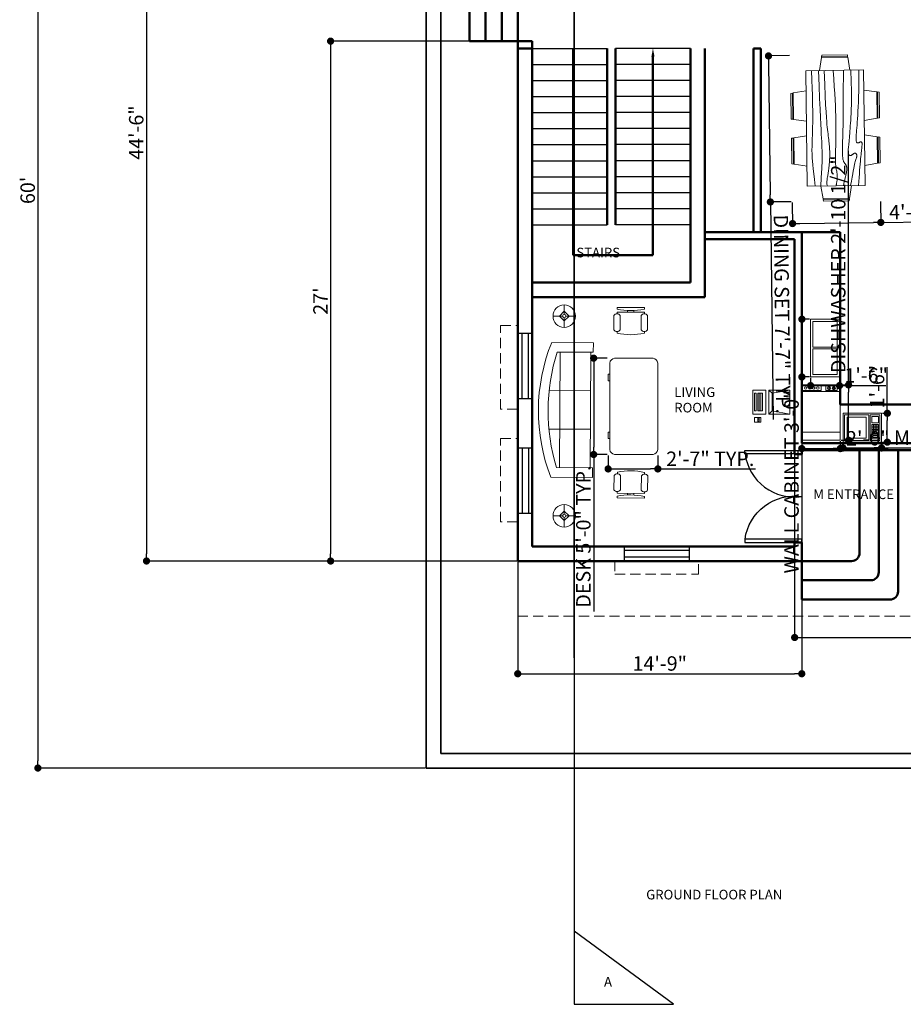
# Model space of a CAD drawing. Units: inches. Extents: x 2050 to 6806, y 2092 to 5743.
# Tile 1 of 8: x 2050 to 2600, y 2092 to 2706. Entities that reach past the tile are written whole.
import ezdxf

# ---------------------------------------------------------------- set-up
doc = ezdxf.new("R2010")
doc.units = ezdxf.units.IN
doc.linetypes.add('HIDDEN', pattern=[9.525, 6.35, -3.175])
for name, color, linetype, lineweight in [('A-ANNO-DIMS', 2, 'Continuous', 18), ('A-ANNO-SYMB', 1, 'Continuous', 25), ('A-ANNO-TEXT', 7, 'Continuous', 25), ('A-AREA-IDEN', 7, 'Continuous', 18), ('A-DOOR', 2, 'Continuous', 25), ('A-FLOR-FIXT', 4, 'Continuous', 18), ('A-FLOR-OVHD', 30, 'HIDDEN', 18), ('A-FLOR-STRS', 3, 'Continuous', 25), ('A-FURN', 5, 'Continuous', 18), ('A-GLAZ', 6, 'Continuous', 25), ('A-WALL', 7, 'Continuous', 50), ('C-PROP', 90, 'Continuous', 35)]:
    doc.layers.add(name, color=color, linetype=linetype, lineweight=lineweight)
doc.styles.get("Standard").update_dxf_attribs({"font": 'arial.ttf'})
doc.dimstyles.new('ISO-25', dxfattribs={"dimtxt": 9, "dimasz": 4.5, "dimexe": 1.25, "dimexo": 0.625, "dimtad": 1, "dimdec": 1, "dimlunit": 4, "dimtxsty": 'Standard', "dimblk": 'DOT', "dimcen": 2.5, "dimadec": 0, "dimazin": 0, "dimtfac": 1, "dimtdec": 1, "dimtmove": 0, "dimatfit": 3, "dimldrblk": 'ARCHTICK', "dimfxl": 1, "dimarcsym": 0})

# ---------------------------------------------------------------- blocks, each defined once
blk = doc.blocks.new('Dining Set - 36 x 72 in.')
for p, q in [((-22.2343, 26.00059), (-23.4847, 17.99762)), ((-22.2304, 26), (-5.7608, 26)), ((-22, 27.5), (-22.1562, 26.50042)), ((-5.8416, 26.5), (-22.1534, 26.5)), ((-22, 27.5), (-6, 27.5)), ((-5.8437, 26.49966), (-6, 27.5)), ((-4.5152, 17.99762), (-5.7655, 25.99926)), ((5.7657, 26.00059), (4.5153, 17.99762)), ((5.7696, 26), (22.2392, 26)), ((6, 27.5), (5.8438, 26.50042)), ((22.1584, 26.5), (5.8466, 26.5)), ((6, 27.5), (22, 27.5)), ((22.1563, 26.49966), (22, 27.5)), ((23.4848, 17.99762), (22.2345, 25.99926)), ((36, 18), (-36, 18)), ((-36, 18), (-36, -18)), ((36, -18), (36, 18)), ((-45.5, 8), (-44.5004, 8.15617)), ((-45.5, 8), (-45.5, -8)), ((-44.5, -8.15843), (-44.5, 8.15338)), ((-44.0006, 8.23428), (-35.9976, 9.48474)), ((-44, 8.23041), (-44, -8.23915)), ((44.0006, 8.23428), (35.9976, 9.48474)), ((44, 8.23041), (44, -8.23915)), ((44.5, -8.15843), (44.5, 8.15338)), ((45.5, 8), (44.5005, 8.15617)), ((45.5, 8), (45.5, -8)), ((-44.4997, -8.15631), (-45.5, -8)), ((-35.9976, -9.48476), (-43.9993, -8.2345)), ((35.9976, -9.48476), (43.9993, -8.2345)), ((44.4997, -8.15631), (45.5, -8)), ((-36, -18), (36, -18)), ((-22.2343, -26.0006), (-23.4847, -17.99762)), ((-4.5152, -17.99762), (-5.7655, -25.99928)), ((5.7657, -26.0006), (4.5153, -17.99762)), ((23.4848, -17.99762), (22.2345, -25.99928)), ((-22.2304, -26), (-5.7608, -26)), ((-22, -27.5), (-22.1562, -26.50044)), ((-5.8416, -26.5), (-22.1534, -26.5)), ((-22, -27.5), (-6, -27.5)), ((-5.8437, -26.49967), (-6, -27.5)), ((5.7696, -26), (22.2392, -26)), ((6, -27.5), (5.8438, -26.50044)), ((22.1584, -26.5), (5.8466, -26.5)), ((6, -27.5), (22, -27.5)), ((22.1563, -26.49967), (22, -27.5))]:
    blk.add_line(p, q)
for points in [[(-36, 15), (-31.1772, 14.97754), (-26.8079, 14.91406), (-22.8538, 14.81543), (-19.276, 14.6875), (-16.0362, 14.53613), (-13.0957, 14.36718), (-10.4159, 14.18652), (-7.9583, 14), (-5.6904, 13.81315), (-3.6035, 13.63021), (-1.6954, 13.45508), (0.0365, 13.29166), (1.5945, 13.14388), (2.9811, 13.01562), (4.1988, 12.9108), (5.25, 12.83333), (6.1393, 12.78613), (6.8802, 12.76823), (7.4883, 12.77767), (7.9792, 12.8125), (8.3685, 12.87077), (8.6719, 12.95052), (8.9049, 13.0498), (9.0833, 13.16666), (9.2205, 13.29899), (9.3216, 13.44401), (9.3895, 13.59879), (9.4271, 13.76041), (9.4373, 13.92594), (9.4232, 14.09245), (9.3875, 14.257), (9.3333, 14.41666), (9.2638, 14.56917), (9.1836, 14.71484), (9.0975, 14.85465), (9.0104, 14.98958), (8.9272, 15.1206), (8.8529, 15.2487), (8.7922, 15.37483), (8.75, 15.5), (8.7305, 15.62467), (8.7344, 15.74739), (8.7617, 15.86621), (8.8125, 15.97916), (8.8867, 16.08431), (8.9844, 16.17968), (9.1055, 16.26334), (9.25, 16.33333), (9.4189, 16.38802), (9.6172, 16.42708), (9.8506, 16.45052), (10.125, 16.45833), (10.4463, 16.45052), (10.8203, 16.42708), (11.2529, 16.38802), (11.75, 16.33333), (12.3184, 16.26318), (12.9694, 16.17838), (13.7151, 16.07991), (14.5677, 15.96875), (15.5395, 15.84586), (16.6426, 15.71224), (17.8893, 15.56884), (19.2917, 15.41666), (20.859, 15.25667), (22.5879, 15.08984), (24.4721, 14.91715), (26.5052, 14.73958), (28.6809, 14.5581), (30.9929, 14.3737), (33.4347, 14.18733), (36, 14)], [(-36, 10), (-28.9766, 10.14274), (-23.1725, 10.20442), (-18.4241, 10.19775), (-14.5677, 10.13541), (-11.4399, 10.03011), (-8.877, 9.89453), (-6.7154, 9.74137), (-4.7917, 9.58333), (-2.9698, 9.43082), (-1.2246, 9.28515), (0.4415, 9.14534), (2.026, 9.01041), (3.5266, 8.87939), (4.9408, 8.7513), (6.266, 8.62516), (7.5, 8.5), (8.6411, 8.37549), (9.6914, 8.2539), (10.6538, 8.13818), (11.5312, 8.03125), (12.3267, 7.93603), (13.043, 7.85547), (13.6831, 7.79248), (14.25, 7.75), (14.7471, 7.7303), (15.1797, 7.73307), (15.5537, 7.75732), (15.875, 7.80208), (16.1494, 7.86637), (16.3828, 7.94922), (16.5811, 8.04964), (16.75, 8.16666), (16.8944, 8.29915), (17.0143, 8.44531), (17.1089, 8.60319), (17.1771, 8.77083), (17.218, 8.94629), (17.2305, 9.1276), (17.2137, 9.31282), (17.1667, 9.5), (17.0895, 9.6875), (16.987, 9.875), (16.8649, 10.0625), (16.7292, 10.25), (16.5856, 10.4375), (16.4401, 10.625), (16.2985, 10.8125), (16.1667, 11), (16.05, 11.18733), (15.9518, 11.3737), (15.8752, 11.5581), (15.8229, 11.73958), (15.798, 11.91715), (15.8034, 12.08984), (15.842, 12.25667), (15.9167, 12.41666), (16.0295, 12.56836), (16.1784, 12.70833), (16.3605, 12.83268), (16.5729, 12.9375), (16.8127, 13.01888), (17.0768, 13.07291), (17.3625, 13.0957), (17.6667, 13.08333), (17.9894, 13.03312), (18.3418, 12.94726), (18.7382, 12.82918), (19.1927, 12.68229), (19.7195, 12.51001), (20.3327, 12.31575), (21.0465, 12.10294), (21.875, 11.875), (22.8357, 11.63354), (23.959, 11.37304), (25.2786, 11.08618), (26.8282, 10.76562), (28.6414, 10.40405), (30.752, 9.99414), (33.1936, 9.52856), (36, 9)], [(-36, 5.5), (-30.7157, 5.3348), (-26.069, 5.20963), (-21.9946, 5.11767), (-18.4271, 5.05208), (-15.3009, 5.00602), (-12.5508, 4.97265), (-10.1112, 4.94515), (-7.9167, 4.91666), (-5.909, 4.88167), (-4.0586, 4.83984), (-2.3429, 4.79215), (-0.7396, 4.73958), (0.7739, 4.6831), (2.22, 4.6237), (3.6213, 4.56233), (5, 4.5), (6.373, 4.43782), (7.7344, 4.3776), (9.0723, 4.32129), (10.375, 4.27083), (11.6309, 4.22819), (12.8281, 4.19531), (13.9551, 4.17415), (15, 4.16666), (15.954, 4.17448), (16.819, 4.19791), (17.6001, 4.23698), (18.3021, 4.29166), (18.9299, 4.36198), (19.4883, 4.44791), (19.9823, 4.54948), (20.4167, 4.66666), (20.7969, 4.79899), (21.1302, 4.94401), (21.4245, 5.09879), (21.6875, 5.26041), (21.9271, 5.42594), (22.1511, 5.59245), (22.3672, 5.757), (22.5834, 5.91666), (22.8065, 6.06868), (23.0404, 6.21093), (23.2879, 6.34147), (23.5521, 6.45833), (23.8358, 6.55957), (24.142, 6.64323), (24.4735, 6.70735), (24.8334, 6.75), (25.2235, 6.76969), (25.642, 6.76692), (26.0858, 6.74267), (26.5521, 6.69791), (27.0379, 6.63362), (27.5404, 6.55078), (28.0565, 6.45036), (28.5834, 6.33333), (29.1242, 6.19987), (29.7071, 6.04687), (30.3661, 5.87044), (31.1354, 5.66666), (32.0493, 5.43164), (33.142, 5.16146), (34.4475, 4.85221), (36, 4.5)], [(-36, -1), (-30.7915, -0.6591), (-26.0195, -0.38216), (-21.6519, -0.16284), (-17.6563, 0.00521), (-14.0005, 0.12833), (-10.6523, 0.21289), (-7.5796, 0.26522), (-4.75, 0.29166), (-2.134, 0.29793), (0.2878, 0.28711), (2.5317, 0.26163), (4.6146, 0.22396), (6.5529, 0.17651), (8.3633, 0.12174), (10.0623, 0.06209), (11.6667, 0), (13.1899, -0.06201), (14.6341, -0.1211), (15.9982, -0.17432), (17.2813, -0.21875), (18.4823, -0.25147), (19.6003, -0.26953), (20.6343, -0.27002), (21.5834, -0.25), (22.4481, -0.20768), (23.2357, -0.14584), (23.9549, -0.06836), (24.6146, 0.02083), (25.2235, 0.11784), (25.7904, 0.21875), (26.3241, 0.31966), (26.8334, 0.41666), (27.3265, 0.50618), (27.8099, 0.58593), (28.2894, 0.65397), (28.7709, 0.70833), (29.2601, 0.74707), (29.763, 0.76823), (30.2855, 0.76985), (30.8334, 0.75), (31.4088, 0.70784), (31.9994, 0.64713), (32.589, 0.57275), (33.1615, 0.48958), (33.7008, 0.4025), (34.1908, 0.3164), (34.6153, 0.23616), (34.9584, 0.16666), (35.2099, 0.11165), (35.3848, 0.07031), (35.504, 0.04069), (35.5886, 0.02083), (35.6594, 0.00879), (35.7377, 0.0026), (35.8442, 0.00032), (36, 0)], [(-36, -6.5), (-27.1843, -6.31267), (-20.084, -6.1263), (-14.469, -5.9419), (-10.1094, -5.76042), (-6.7752, -5.58285), (-4.2363, -5.41016), (-2.2629, -5.24333), (-0.625, -5.08334), (0.8708, -4.93099), (2.2715, -4.78646), (3.5872, -4.64974), (4.8281, -4.52084), (6.0046, -4.39974), (7.127, -4.28646), (8.2053, -4.18099), (9.25, -4.08334), (10.2705, -3.99382), (11.2734, -3.91407), (12.2647, -3.84603), (13.25, -3.79167), (14.2354, -3.75293), (15.2266, -3.73177), (16.2295, -3.73015), (17.25, -3.75), (18.2912, -3.79248), (19.3451, -3.85547), (20.4009, -3.93604), (21.4479, -4.03125), (22.4754, -4.13819), (23.4727, -4.25391), (24.4289, -4.37549), (25.3334, -4.5), (26.1785, -4.62492), (26.9694, -4.74935), (27.7145, -4.87281), (28.4219, -4.99479), (29.1, -5.11483), (29.7572, -5.23242), (30.4016, -5.34709), (31.0417, -5.45834), (31.6837, -5.56437), (32.3262, -5.65821), (32.9658, -5.73153), (33.599, -5.77604), (34.2224, -5.78345), (34.8327, -5.74545), (35.4264, -5.65373), (36, -5.5)], [(-36, -10), (-26.4022, -9.81299), (-18.4675, -9.62891), (-11.9839, -9.45069), (-6.7396, -9.28125), (-2.5226, -9.12354), (0.8789, -8.98047), (3.6769, -8.85498), (6.0833, -8.75), (8.2767, -8.66765), (10.3021, -8.60677), (12.1712, -8.56543), (13.8958, -8.54167), (15.4876, -8.53353), (16.9583, -8.53907), (18.3197, -8.55632), (19.5834, -8.58334), (20.7616, -8.61841), (21.8685, -8.66081), (22.9188, -8.71004), (23.9271, -8.76563), (24.9081, -8.82707), (25.8763, -8.89388), (26.8465, -8.96558), (27.8334, -9.04167), (28.8474, -9.12118), (29.8828, -9.20117), (30.93, -9.27824), (31.9792, -9.34896), (33.0205, -9.40991), (34.0443, -9.45768), (35.0407, -9.48885), (36, -9.5)], [(-36, -14.5), (-30.0881, -14.33513), (-25.0332, -14.21224), (-20.7312, -14.12647), (-17.0781, -14.07292), (-13.97, -14.04671), (-11.3027, -14.04297), (-8.9724, -14.05681), (-6.875, -14.08334), (-4.9224, -14.11833), (-3.0905, -14.16016), (-1.3709, -14.20785), (0.2448, -14.26042), (1.7647, -14.3169), (3.1973, -14.3763), (4.5507, -14.43767), (5.8333, -14.5), (7.0554, -14.5621), (8.235, -14.62175), (9.3922, -14.67652), (10.5469, -14.72396), (11.7192, -14.76164), (12.929, -14.78711), (14.1965, -14.79794), (15.5417, -14.79167), (16.9933, -14.76424), (18.6152, -14.70508), (20.4804, -14.60197), (22.6615, -14.44271), (25.2312, -14.21509), (28.2624, -13.9069), (31.8277, -13.50594), (36, -13)]]:
    blk.add_lwpolyline(points)
blk = doc.blocks.new('Microwave')
for p, q in [((18, 10), (22, 10)), ((22, 9), (18, 9)), ((18, 8), (22, 8)), ((22, 7), (18, 7)), ((19, 7), (19, 11)), ((19, 6), (19, 7)), ((20, 11), (20, 7)), ((20, 7), (20, 6)), ((21, 7), (21, 11)), ((20, 6), (18, 6))]:
    blk.add_line(p, q)
for points in [[(0, 0), (0, 18), (24, 18), (24, 0)], [(1, 1), (1, 17), (16, 17), (16, 1)], [(2.5, 2.5), (2.5, 15.5), (14.5, 15.5), (14.5, 2.5)], [(17, 1), (17, 17), (23, 17), (23, 1)], [(18, 12), (18, 16), (22, 16), (22, 12)], [(18, 2), (18, 11), (22, 11), (22, 2)], [(18.5, 4.5), (18.5, 5.5), (21.5, 5.5), (21.5, 4.5)], [(18.5, 3), (18.5, 4), (21.5, 4), (21.5, 3)]]:
    blk.add_lwpolyline(points, close=True)
blk = doc.blocks.new('Dishwasher')
for p, q in [((16, 32.5), (16.75, 32.5)), ((16.5, 32), (16.2942, 31.7942)), ((16.3156, 33.1843), (16.5, 33)), ((17, 32.75), (17, 33.5)), ((17, 32.25), (17, 31.5)), ((18, 32.5), (17.25, 32.5)), ((17.5, 33), (17.6938, 33.1938)), ((17.7061, 31.7939), (17.5, 32)), ((19, 32.5), (19.75, 32.5)), ((19.5, 32), (19.2942, 31.7942)), ((19.3156, 33.1843), (19.5, 33)), ((20, 32.75), (20, 33.5)), ((20, 32.25), (20, 31.5)), ((21, 32.5), (20.25, 32.5)), ((20.5, 33), (20.6938, 33.1938)), ((20.7061, 31.7939), (20.5, 32)), ((24, 30.5), (0, 30.5)), ((0, 5), (24, 5))]:
    blk.add_line(p, q)
for points in [[(0, 0), (0, 34.5), (24, 34.5), (24, 0)], [(0.5, 31), (0.5, 34), (12, 34), (12, 31)], [(15, 31), (15, 34), (22, 34), (22, 31)]]:
    blk.add_lwpolyline(points, close=True)
for centre, radius in [((2.5, 32.5), 0.75), ((5, 32.5), 0.75), ((7.5, 32.5), 0.75), ((10, 32.5), 0.75), ((17, 32.5), 1), ((20, 32.5), 1)]:
    blk.add_circle(centre, radius)
blk = doc.blocks.new('Wall Cabinet - 18 x 36 in front')
for p, q in [((17.5, -1.5), (17.5, -16.5)), ((18.5, -16.5), (18.5, -1.5))]:
    blk.add_line(p, q)
blk.add_lwpolyline([(0, -18), (0, 0), (36, 0), (36, -18)], close=True)
for points in [[(17.5, -16.5), (1.5, -16.5), (1.5, -1.5), (17.5, -1.5)], [(18.5, -1.5), (34.5, -1.5), (34.5, -16.5), (18.5, -16.5)]]:
    blk.add_lwpolyline(points)
blk = doc.blocks.new('Sofa - Roundback 7 ft.')
for p, q in [((-36.000027, -34), (-36.000027, -11.4696)), ((-12.00002, -32.4421), (-12.00003, -6.5971)), ((11.99997, -32.4421), (11.99998, -6.5971)), ((35.99998, -34), (35.99998, -11.4696)), ((-35.999844, -13.3819), (35.9998, -13.3819)), ((-36.000027, -32.4421), (35.99998, -32.4421))]:
    blk.add_line(p, q)
for points in [[(-36.000027, -34), (-42.000027, -34), (-42.000027, -8)], [(41.99998, -8), (41.99998, -34), (35.99998, -34)]]:
    blk.add_lwpolyline(points)
for centre, radius, start, end in [((0, -114.25), 114.25, 68.43141, 111.5686), ((-0.00001, -127.1968), 121.1968, 72.72033, 107.2797)]:
    blk.add_arc(centre, radius, start, end)
blk = doc.blocks.new('Desk - 30 x 60 in.')
for p, q in [((-26.999995, 0), (26.999995, 0)), ((-29.999995, -27), (-29.999995, -3)), ((29.999995, -3), (29.999995, -27)), ((26.999995, -30), (-26.999995, -30)), ((-20.000005, -30), (-20.000005, -31)), ((-16.000005, -31), (-16.000005, -30)), ((15.999995, -31), (15.999995, -30)), ((19.999995, -30), (19.999995, -31)), ((-20.000005, -31), (-16.000005, -31)), ((19.999995, -31), (15.999995, -31))]:
    blk.add_line(p, q)
for centre, start, end in [((-26.499995, -3.5), 98.1301, 171.8699), ((26.499995, -3.5), 8.130102, 81.8699), ((-26.499995, -26.5), 188.1301, 261.8699), ((26.499995, -26.5), 278.1301, 351.8699)]:
    blk.add_arc(centre, 3.535534, start, end)
blk = doc.blocks.new('Chair - Desk')
for p, q in [((-8.5, 0), (-8.5, -1)), ((-8.5, 0), (8.5, 0)), ((8.5, 0), (8.5, -1)), ((-10.5, -5), (-10.5, -14)), ((-8.5, -3), (-8.5, -4)), ((-8.5, -3), (8.5, -3)), ((-6.5, -14), (-6.5, -5)), ((-2, -3), (-2, -1.9355)), ((2, -1.9576), (2, -3)), ((6.5, -5), (6.5, -14)), ((8.5, -3), (8.5, -4)), ((10.5, -14), (10.5, -5)), ((-8.5, -15), (-8.5, -16)), ((8.5, -15), (8.5, -16))]:
    blk.add_line(p, q)
for centre, radius, start, end in [((-8.5, -6.5), 2.5, 36.8699, 143.1301), ((0, 34.625), 36.625, 256.5803, 283.4197), ((8.5, -6.5), 2.5, 36.8699, 143.1301), ((-8.5, -12.5), 2.5, 216.8699, 323.1301), ((0, 19.625), 36.625, 256.5803, 283.4197), ((8.5, -12.5), 2.5, 216.8699, 323.1301)]:
    blk.add_arc(centre, radius, start, end)
blk = doc.blocks.new('Lamp - Table')
for p, q in [((0, 7), (0, 1)), ((-1, 0), (-7, 0)), ((0, 3), (-3, 0)), ((-3, 0), (0, -3)), ((3, 0), (0, 3)), ((0, -3), (3, 0)), ((1, 0), (7, 0)), ((0, -1), (0, -7))]:
    blk.add_line(p, q)
for radius in [7, 1]:
    blk.add_circle((0, 0), radius)
blk = doc.blocks.new('Computer Terminal')
for p, q in [((-10, 11.5), (5, 11.5)), ((-8, 0.5), (-10, 11.5)), ((-10, -1.5), (-10, 11.5)), ((5, 11.5), (3, 0.5)), ((5, 11.5), (5, -1.5)), ((-10, -1.5), (-8, 0.5)), ((3, 0.5), (-8, 0.5)), ((3, 0.5), (5, -1.5)), ((5, -1.5), (-10, -1.5)), ((-10, -11.5), (-10, -3.5)), ((-10, -3.5), (5, -3.5)), ((-8, -5.5), (-8, -8.5)), ((3, -5.5), (-8, -5.5)), ((3, -8.5), (3, -5.5)), ((5, -3.5), (5, -11.5)), ((5, -11.5), (-10, -11.5)), ((3, -6.5), (-8, -6.5)), ((-8, -7.5), (3, -7.5)), ((-8, -8.5), (3, -8.5)), ((-8, -9.5), (-8, -10.5)), ((3, -9.5), (-8, -9.5)), ((-8, -10.5), (3, -10.5)), ((3, -10.5), (3, -9.5)), ((10, -6.5), (7, -6.5)), ((7, -6.5), (7, -10.5)), ((7, -10.5), (10, -10.5)), ((9.5, -7.5), (7.5, -7.5)), ((7.5, -7.5), (7.5, -8.5)), ((7.5, -8.5), (9.5, -8.5)), ((8.5, -7.5), (8.5, -8.5)), ((9.5, -8.5), (9.5, -7.5)), ((10, -10.5), (10, -6.5))]:
    blk.add_line(p, q)
blk = doc.blocks.new('_Dot')
at = {"color": 0, "linetype": 'ByBlock', "lineweight": -2}
blk.add_line((-0.5, 0), (-1, 0), dxfattribs=at)
at = {"color": 0, "linetype": 'ByBlock', "const_width": 0.5}
blk.add_lwpolyline([(-0.25, 0, 1), (0.25, 0, 1)], format="xyb", close=True, dxfattribs=at)
blk = doc.blocks.new('*D27')
at = {"layer": 'A-ANNO-DIMS', "color": 0, "lineweight": -2, "transparency": 16777216}
for p, q in [((2302.28, 2959.24), (2059.63, 2959.24)), ((2060.88, 2954.74), (2060.88, 2243.74)), ((2302.28, 2239.24), (2059.63, 2239.24))]:
    blk.add_line(p, q, dxfattribs=at)
at = {"layer": 'Defpoints', "color": 0, "transparency": 16777216}
for p in [(2302.91, 2959.24), (2060.88, 2239.24), (2302.91, 2239.24)]:
    blk.add_point(p, dxfattribs=at)
at = {"layer": 'A-ANNO-DIMS', "color": 0, "lineweight": -2, "transparency": 16777216, "xscale": 4.5, "yscale": 4.5, "zscale": 4.5}
for p, rotation in [((2060.88, 2959.24), 90), ((2060.88, 2239.24), 270)]:
    blk.add_blockref('_Dot', p, dxfattribs=dict(at, rotation=rotation))
at = {"layer": 'A-ANNO-DIMS', "color": 0, "transparency": 16777216, "insert": (2055.66, 2599.24), "char_height": 9, "attachment_point": 5, "rotation": 90}
blk.add_mtext("60'", dxfattribs=at)
blk = doc.blocks.new('_ArchTick')
at = {"color": 0, "linetype": 'ByBlock', "const_width": 0.15}
blk.add_lwpolyline([(-0.5, -0.5), (0.5, 0.5)], dxfattribs=at)
blk = doc.blocks.new('*D28')
at = {"layer": 'A-ANNO-DIMS', "color": 0, "lineweight": -2, "transparency": 16777216}
for p, q in [((2359.28, 2902.24), (2127.3, 2902.24)), ((2128.55, 2897.74), (2128.55, 2372.74)), ((2359.28, 2368.24), (2127.3, 2368.24))]:
    blk.add_line(p, q, dxfattribs=at)
at = {"layer": 'Defpoints', "color": 0, "transparency": 16777216}
for p in [(2359.91, 2902.24), (2128.55, 2368.24), (2359.91, 2368.24)]:
    blk.add_point(p, dxfattribs=at)
at = {"layer": 'A-ANNO-DIMS', "color": 0, "lineweight": -2, "transparency": 16777216, "xscale": 4.5, "yscale": 4.5, "zscale": 4.5}
for p, rotation in [((2128.55, 2902.24), 90), ((2128.55, 2368.24), 270)]:
    blk.add_blockref('_Dot', p, dxfattribs=dict(at, rotation=rotation))
at = {"layer": 'A-ANNO-DIMS', "color": 0, "transparency": 16777216, "insert": (2123.33, 2635.24), "char_height": 9, "attachment_point": 5, "rotation": 90}
blk.add_mtext('44\'-6"', dxfattribs=at)
blk = doc.blocks.new('*D30')
at = {"layer": 'A-ANNO-DIMS', "color": 0, "lineweight": -2, "transparency": 16777216}
for p, q in [((2359.28, 2692.24), (2242.04, 2692.24)), ((2243.29, 2687.74), (2243.29, 2372.74)), ((2359.28, 2368.24), (2242.04, 2368.24))]:
    blk.add_line(p, q, dxfattribs=at)
at = {"layer": 'Defpoints', "color": 0, "transparency": 16777216}
for p in [(2359.91, 2692.24), (2243.29, 2368.24), (2359.91, 2368.24)]:
    blk.add_point(p, dxfattribs=at)
at = {"layer": 'A-ANNO-DIMS', "color": 0, "lineweight": -2, "transparency": 16777216, "xscale": 4.5, "yscale": 4.5, "zscale": 4.5}
for p, rotation in [((2243.29, 2692.24), 90), ((2243.29, 2368.24), 270)]:
    blk.add_blockref('_Dot', p, dxfattribs=dict(at, rotation=rotation))
at = {"layer": 'A-ANNO-DIMS', "color": 0, "transparency": 16777216, "insert": (2238.15, 2530.24), "char_height": 9, "attachment_point": 5, "rotation": 90}
blk.add_mtext("27'", dxfattribs=at)
blk = doc.blocks.new('*D31')
at = {"layer": 'A-ANNO-DIMS', "color": 0, "lineweight": -2, "transparency": 16777216}
for p, q in [((2359.91, 2367.61), (2359.91, 2296.75)), ((2536.91, 2367.61), (2536.91, 2296.75)), ((2364.41, 2298), (2532.41, 2298))]:
    blk.add_line(p, q, dxfattribs=at)
at = {"layer": 'Defpoints', "color": 0, "transparency": 16777216}
for p in [(2359.91, 2368.24), (2536.91, 2368.24), (2536.91, 2298)]:
    blk.add_point(p, dxfattribs=at)
at = {"layer": 'A-ANNO-DIMS', "color": 0, "lineweight": -2, "transparency": 16777216, "xscale": 4.5, "yscale": 4.5, "zscale": 4.5, "rotation": 180}
blk.add_blockref('_Dot', (2359.91, 2298), dxfattribs=at)
at = {"layer": 'A-ANNO-DIMS', "color": 0, "lineweight": -2, "transparency": 16777216, "xscale": 4.5, "yscale": 4.5, "zscale": 4.5}
blk.add_blockref('_Dot', (2536.91, 2298), dxfattribs=at)
at = {"layer": 'A-ANNO-DIMS', "color": 0, "transparency": 16777216, "insert": (2448.41, 2303.22), "char_height": 9, "attachment_point": 5}
blk.add_mtext('14\'-9"', dxfattribs=at)
blk = doc.blocks.new('*D32')
at = {"layer": 'A-ANNO-DIMS', "color": 0, "lineweight": -2, "transparency": 16777216}
for p, q in [((2532.41, 2436.47), (2532.47, 2319.32)), ((2821.91, 2436.61), (2821.97, 2319.47)), ((2536.97, 2320.57), (2817.47, 2320.71))]:
    blk.add_line(p, q, dxfattribs=at)
at = {"layer": 'Defpoints', "color": 0, "transparency": 16777216}
for p in [(2532.41, 2437.09), (2821.91, 2437.24), (2821.97, 2320.72)]:
    blk.add_point(p, dxfattribs=at)
at = {"layer": 'A-ANNO-DIMS', "color": 0, "lineweight": -2, "transparency": 16777216, "xscale": 4.5, "yscale": 4.5, "zscale": 4.5}
for p, rotation in [((2532.47, 2320.57), 180.0291193537901), ((2821.97, 2320.72), 0.029119353790171)]:
    blk.add_blockref('_Dot', p, dxfattribs=dict(at, rotation=rotation))
at = {"layer": 'A-ANNO-DIMS', "color": 0, "transparency": 16777216, "insert": (2677.21, 2331.81), "char_height": 9, "attachment_point": 5, "rotation": 0.02912}
blk.add_mtext('24\'-1{\\H1x;\\S1/2;}"', dxfattribs=at)
blk = doc.blocks.new('DOOR-750')
blk.add_lwpolyline([(28.97, 0), (26.83, 0), (26.83, 35.38), (28.97, 35.38)], close=True)
blk.add_arc((31.25, 4.42), 31.27, 98.12333, 188.12333)
blk = doc.blocks.new('DOOR-DOUBLE')
blk.add_lwpolyline([(35.38, 28.96), (35.38, 26.82), (0, 26.82), (0, 28.96)], close=True)
blk.add_lwpolyline([(35.38, 28.96), (35.38, 26.82), (0, 26.82), (0, 28.96)], close=True)
blk.add_arc((30.96, 31.24), 31.27, 188.12333, 278.12333)
blk.add_arc((30.96, 31.24), 31.27, 188.12333, 278.12333)
blk = doc.blocks.new('WIN-1050')
for p, q in [((0, 40.58), (9, 40.58)), ((2.5, 0), (2.5, 40.58)), ((6.5, 0), (6.5, 40.58)), ((0, 0), (9, 0))]:
    blk.add_line(p, q)
blk = doc.blocks.new('SUNSHADE-A')
for p, q in [((0, 52.08), (10.45, 52.08)), ((10.45, 52.08), (10.45, 0)), ((10.45, 0), (0, 0))]:
    blk.add_line(p, q)
blk = doc.blocks.new('SUNSHADE-C')
for p, q in [((0, 8.26), (0, 0)), ((52.07, 0), (52.07, 8.25)), ((0, 0), (52.07, 0))]:
    blk.add_line(p, q)
blk = doc.blocks.new('*D93')
at = {"layer": 'A-ANNO-DIMS', "color": 0, "lineweight": -2, "transparency": 16777216}
for p, q in [((2529.19, 2683.19), (2514.92, 2683)), ((2516.23, 2678.52), (2517.28, 2596.53)), ((2530.36, 2592.19), (2516.09, 2592.01)), ((2517.34, 2592.03), (2519.07, 2456.43))]:
    blk.add_line(p, q, dxfattribs=at)
at = {"layer": 'Defpoints', "color": 0, "transparency": 16777216}
for p in [(2529.82, 2683.2), (2517.34, 2592.03), (2530.98, 2592.2)]:
    blk.add_point(p, dxfattribs=at)
at = {"layer": 'A-ANNO-DIMS', "color": 0, "lineweight": -2, "transparency": 16777216, "xscale": 4.5, "yscale": 4.5, "zscale": 4.5}
for p, rotation in [((2516.17, 2683.02), 90.73372649959308), ((2517.34, 2592.03), 270.733726499593)]:
    blk.add_blockref('_Dot', p, dxfattribs=dict(at, rotation=rotation))
at = {"layer": 'A-ANNO-DIMS', "color": 0, "transparency": 16777216, "insert": (2523.51, 2522.05), "char_height": 9, "attachment_point": 5, "rotation": 270.73373}
blk.add_mtext('DINING SET 7\'-7" TYP.', dxfattribs=at)
blk = doc.blocks.new('*D94')
at = {"layer": 'A-ANNO-DIMS', "color": 0, "lineweight": -2, "transparency": 16777216}
for p, q in [((2530.99, 2591.58), (2531.18, 2577.3)), ((2585.99, 2592.28), (2586.17, 2578.01)), ((2535.66, 2578.61), (2581.66, 2579.2)), ((2586.16, 2579.26), (2647.12, 2580.04))]:
    blk.add_line(p, q, dxfattribs=at)
at = {"layer": 'Defpoints', "color": 0, "transparency": 16777216}
for p in [(2530.98, 2592.2), (2585.98, 2592.91), (2586.16, 2579.26)]:
    blk.add_point(p, dxfattribs=at)
at = {"layer": 'A-ANNO-DIMS', "color": 0, "lineweight": -2, "transparency": 16777216, "xscale": 4.5, "yscale": 4.5, "zscale": 4.5}
for p, rotation in [((2531.16, 2578.55), 180.7337264995931), ((2586.16, 2579.26), 0.7337264995931003)]:
    blk.add_blockref('_Dot', p, dxfattribs=dict(at, rotation=rotation))
at = {"layer": 'A-ANNO-DIMS', "color": 0, "transparency": 16777216, "insert": (2618.82, 2584.8), "char_height": 9, "attachment_point": 5, "rotation": 0.73373}
blk.add_mtext('4\'-7" TYP.', dxfattribs=at)
blk = doc.blocks.new('*D97')
at = {"layer": 'A-ANNO-DIMS', "color": 0, "lineweight": -2, "transparency": 16777216}
for p, q in [((2415.62, 2494.64), (2405.99, 2494.64)), ((2407.24, 2490.14), (2407.24, 2439.14)), ((2415.62, 2434.64), (2405.99, 2434.64)), ((2407.24, 2434.64), (2407.24, 2336.75))]:
    blk.add_line(p, q, dxfattribs=at)
at = {"layer": 'Defpoints', "color": 0, "transparency": 16777216}
for p in [(2416.24, 2494.64), (2407.24, 2434.64), (2416.24, 2434.64)]:
    blk.add_point(p, dxfattribs=at)
at = {"layer": 'A-ANNO-DIMS', "color": 0, "lineweight": -2, "transparency": 16777216, "xscale": 4.5, "yscale": 4.5, "zscale": 4.5}
for p, rotation in [((2407.24, 2494.64), 90), ((2407.24, 2434.64), 270)]:
    blk.add_blockref('_Dot', p, dxfattribs=dict(at, rotation=rotation))
at = {"layer": 'A-ANNO-DIMS', "color": 0, "transparency": 16777216, "insert": (2401.96, 2383.45), "char_height": 9, "attachment_point": 5, "rotation": 90}
blk.add_mtext('DESK 5\'-0" TYP.', dxfattribs=at)
blk = doc.blocks.new('*D98')
at = {"layer": 'A-ANNO-DIMS', "color": 0, "lineweight": -2, "transparency": 16777216}
for p, q in [((2416.24, 2434.02), (2416.24, 2424.39)), ((2447.24, 2434.02), (2447.24, 2424.39)), ((2420.74, 2425.64), (2442.74, 2425.64)), ((2447.24, 2425.64), (2508, 2425.64))]:
    blk.add_line(p, q, dxfattribs=at)
at = {"layer": 'Defpoints', "color": 0, "transparency": 16777216}
for p in [(2416.24, 2434.64), (2447.24, 2434.64), (2447.24, 2425.64)]:
    blk.add_point(p, dxfattribs=at)
at = {"layer": 'A-ANNO-DIMS', "color": 0, "lineweight": -2, "transparency": 16777216, "xscale": 4.5, "yscale": 4.5, "zscale": 4.5, "rotation": 180}
blk.add_blockref('_Dot', (2416.24, 2425.64), dxfattribs=at)
at = {"layer": 'A-ANNO-DIMS', "color": 0, "lineweight": -2, "transparency": 16777216, "xscale": 4.5, "yscale": 4.5, "zscale": 4.5}
blk.add_blockref('_Dot', (2447.24, 2425.64), dxfattribs=at)
at = {"layer": 'A-ANNO-DIMS', "color": 0, "transparency": 16777216, "insert": (2479.87, 2430.79), "char_height": 9, "attachment_point": 5}
blk.add_mtext('2\'-7" TYP.', dxfattribs=at)
blk = doc.blocks.new('*D105')
at = {"layer": 'A-ANNO-DIMS', "color": 0, "lineweight": -2, "transparency": 16777216}
for p, q in [((2562.63, 2441.66), (2562.63, 2437.44)), ((2567.13, 2438.69), (2582.13, 2438.69)), ((2586.63, 2441.66), (2586.63, 2437.44)), ((2586.63, 2438.69), (2698.32, 2438.69))]:
    blk.add_line(p, q, dxfattribs=at)
at = {"layer": 'Defpoints', "color": 0, "transparency": 16777216}
for p in [(2562.63, 2442.29), (2586.63, 2442.29), (2586.63, 2438.69)]:
    blk.add_point(p, dxfattribs=at)
at = {"layer": 'A-ANNO-DIMS', "color": 0, "lineweight": -2, "transparency": 16777216, "xscale": 4.5, "yscale": 4.5, "zscale": 4.5, "rotation": 180}
blk.add_blockref('_Dot', (2562.63, 2438.69), dxfattribs=at)
at = {"layer": 'A-ANNO-DIMS', "color": 0, "lineweight": -2, "transparency": 16777216, "xscale": 4.5, "yscale": 4.5, "zscale": 4.5}
blk.add_blockref('_Dot', (2586.63, 2438.69), dxfattribs=at)
at = {"layer": 'A-ANNO-DIMS', "color": 0, "transparency": 16777216, "insert": (2644.72, 2443.97), "char_height": 9, "attachment_point": 5}
blk.add_mtext('MICROWAVE 2\'-0"', dxfattribs=at)
blk = doc.blocks.new('*D106')
at = {"layer": 'A-ANNO-DIMS', "color": 0, "lineweight": -2, "transparency": 16777216}
for p, q in [((2590.23, 2460.29), (2590.23, 2489.12)), ((2587.25, 2460.29), (2591.48, 2460.29)), ((2590.23, 2446.79), (2590.23, 2455.79)), ((2587.25, 2442.29), (2591.48, 2442.29))]:
    blk.add_line(p, q, dxfattribs=at)
at = {"layer": 'Defpoints', "color": 0, "transparency": 16777216}
for p in [(2586.63, 2460.29), (2590.23, 2460.29), (2586.63, 2442.29)]:
    blk.add_point(p, dxfattribs=at)
at = {"layer": 'A-ANNO-DIMS', "color": 0, "lineweight": -2, "transparency": 16777216, "xscale": 4.5, "yscale": 4.5, "zscale": 4.5}
for p, rotation in [((2590.23, 2460.29), 90), ((2590.23, 2442.29), 270)]:
    blk.add_blockref('_Dot', p, dxfattribs=dict(at, rotation=rotation))
at = {"layer": 'A-ANNO-DIMS', "color": 0, "transparency": 16777216, "insert": (2585.01, 2476.95), "char_height": 9, "attachment_point": 5, "rotation": 90}
blk.add_mtext('1\'-6"', dxfattribs=at)
blk = doc.blocks.new('*D107')
at = {"layer": 'A-ANNO-DIMS', "color": 0, "lineweight": -2, "transparency": 16777216}
for p, q in [((2566.08, 2477.99), (2566.08, 2623.89)), ((2561.53, 2477.99), (2567.33, 2477.99)), ((2566.08, 2447.99), (2566.08, 2473.49)), ((2561.53, 2443.49), (2567.33, 2443.49))]:
    blk.add_line(p, q, dxfattribs=at)
at = {"layer": 'Defpoints', "color": 0, "transparency": 16777216}
for p in [(2560.91, 2477.99), (2566.08, 2477.99), (2560.91, 2443.49)]:
    blk.add_point(p, dxfattribs=at)
at = {"layer": 'A-ANNO-DIMS', "color": 0, "lineweight": -2, "transparency": 16777216, "xscale": 4.5, "yscale": 4.5, "zscale": 4.5}
for p, rotation in [((2566.08, 2477.99), 90), ((2566.08, 2443.49), 270)]:
    blk.add_blockref('_Dot', p, dxfattribs=dict(at, rotation=rotation))
at = {"layer": 'A-ANNO-DIMS', "color": 0, "transparency": 16777216, "insert": (2560.81, 2553.19), "char_height": 9, "attachment_point": 5, "rotation": 90}
blk.add_mtext('DISHWASHER 2\'-10 1/2"', dxfattribs=at)
blk = doc.blocks.new('*D108')
at = {"layer": 'A-ANNO-DIMS', "color": 0, "lineweight": -2, "transparency": 16777216}
for p, q in [((2536.91, 2442.86), (2536.91, 2437.06)), ((2560.91, 2442.86), (2560.91, 2437.06)), ((2541.41, 2438.31), (2556.41, 2438.31)), ((2560.91, 2438.31), (2590.74, 2438.31))]:
    blk.add_line(p, q, dxfattribs=at)
at = {"layer": 'Defpoints', "color": 0, "transparency": 16777216}
for p in [(2536.91, 2443.49), (2560.91, 2443.49), (2560.91, 2438.31)]:
    blk.add_point(p, dxfattribs=at)
at = {"layer": 'A-ANNO-DIMS', "color": 0, "lineweight": -2, "transparency": 16777216, "xscale": 4.5, "yscale": 4.5, "zscale": 4.5, "rotation": 180}
blk.add_blockref('_Dot', (2536.91, 2438.31), dxfattribs=at)
at = {"layer": 'A-ANNO-DIMS', "color": 0, "lineweight": -2, "transparency": 16777216, "xscale": 4.5, "yscale": 4.5, "zscale": 4.5}
blk.add_blockref('_Dot', (2560.91, 2438.31), dxfattribs=at)
at = {"layer": 'A-ANNO-DIMS', "color": 0, "transparency": 16777216, "insert": (2578.07, 2443.53), "char_height": 9, "attachment_point": 5}
blk.add_mtext('2\'-0"', dxfattribs=at)
blk = doc.blocks.new('*D109')
at = {"layer": 'A-ANNO-DIMS', "color": 0, "lineweight": -2, "transparency": 16777216}
for p, q in [((2541.77, 2518.94), (2535.75, 2518.94)), ((2537, 2514.44), (2537, 2487.44)), ((2541.77, 2482.94), (2535.75, 2482.94)), ((2537, 2482.94), (2537, 2357.18))]:
    blk.add_line(p, q, dxfattribs=at)
at = {"layer": 'Defpoints', "color": 0, "transparency": 16777216}
for p in [(2542.4, 2518.94), (2537, 2482.94), (2542.4, 2482.94)]:
    blk.add_point(p, dxfattribs=at)
at = {"layer": 'A-ANNO-DIMS', "color": 0, "lineweight": -2, "transparency": 16777216, "xscale": 4.5, "yscale": 4.5, "zscale": 4.5}
for p, rotation in [((2537, 2518.94), 90), ((2537, 2482.94), 270)]:
    blk.add_blockref('_Dot', p, dxfattribs=dict(at, rotation=rotation))
at = {"layer": 'A-ANNO-DIMS', "color": 0, "transparency": 16777216, "insert": (2531.72, 2417.81), "char_height": 9, "attachment_point": 5, "rotation": 90}
blk.add_mtext('WALL CABINET 3\'-0"', dxfattribs=at)
blk = doc.blocks.new('*D110')
at = {"layer": 'A-ANNO-DIMS', "color": 0, "lineweight": -2, "transparency": 16777216}
for p, q in [((2542.4, 2482.32), (2542.4, 2476.29)), ((2560.4, 2482.32), (2560.4, 2476.29)), ((2546.9, 2477.54), (2555.9, 2477.54)), ((2560.4, 2477.54), (2589.22, 2477.54))]:
    blk.add_line(p, q, dxfattribs=at)
at = {"layer": 'Defpoints', "color": 0, "transparency": 16777216}
for p in [(2542.4, 2482.94), (2560.4, 2482.94), (2560.4, 2477.54)]:
    blk.add_point(p, dxfattribs=at)
at = {"layer": 'A-ANNO-DIMS', "color": 0, "lineweight": -2, "transparency": 16777216, "xscale": 4.5, "yscale": 4.5, "zscale": 4.5, "rotation": 180}
blk.add_blockref('_Dot', (2542.4, 2477.54), dxfattribs=at)
at = {"layer": 'A-ANNO-DIMS', "color": 0, "lineweight": -2, "transparency": 16777216, "xscale": 4.5, "yscale": 4.5, "zscale": 4.5}
blk.add_blockref('_Dot', (2560.4, 2477.54), dxfattribs=at)
at = {"layer": 'A-ANNO-DIMS', "color": 0, "transparency": 16777216, "insert": (2577.06, 2482.76), "char_height": 9, "attachment_point": 5}
blk.add_mtext('1\'-6"', dxfattribs=at)

msp = doc.modelspace()

# ---------------------------------------------------------------- linework, layer by layer
at = {"layer": 'A-ANNO-SYMB'}
for p, q in [((2395, 3128.67), (2395, 2091.98)), ((2395, 2307.82), (2395, 3128.67)), ((2456.98, 2091.98), (2395, 2137.51)), ((2395, 2091.98), (2456.98, 2091.98)), ((2456.98, 2091.98), (2456.98, 2091.98))]:
    msp.add_line(p, q, dxfattribs=at)
at = {"layer": 'A-FLOR-OVHD'}
for p, q in [((2359.91, 2368.24), (2359.91, 2333.88)), ((2359.91, 2333.88), (2608.94, 2333.88))]:
    msp.add_line(p, q, dxfattribs=at)
at = {"layer": 'A-FLOR-STRS'}
for p, q in [((2368.91, 2687.74), (2404.91, 2687.74)), ((2368.91, 2687.74), (2415.59, 2687.74)), ((2467.51, 2687.74), (2420.83, 2687.74)), ((2467.51, 2687.74), (2431.51, 2687.74)), ((2368.91, 2677.74), (2415.59, 2677.74)), ((2467.51, 2677.74), (2420.83, 2677.74)), ((2368.91, 2667.74), (2415.59, 2667.74)), ((2467.51, 2667.74), (2420.83, 2667.74)), ((2368.91, 2657.74), (2415.59, 2657.74)), ((2467.51, 2657.74), (2420.83, 2657.74)), ((2368.91, 2647.74), (2415.59, 2647.74)), ((2467.51, 2647.74), (2420.83, 2647.74)), ((2368.91, 2637.74), (2415.59, 2637.74)), ((2467.51, 2637.74), (2420.83, 2637.74)), ((2368.91, 2627.74), (2415.59, 2627.74)), ((2467.51, 2627.74), (2420.83, 2627.74)), ((2368.91, 2617.74), (2415.59, 2617.74)), ((2467.51, 2617.74), (2420.83, 2617.74)), ((2368.91, 2607.74), (2415.59, 2607.74)), ((2467.51, 2607.74), (2420.83, 2607.74)), ((2368.91, 2597.74), (2415.59, 2597.74)), ((2467.51, 2597.74), (2420.83, 2597.74)), ((2368.91, 2587.74), (2415.59, 2587.74)), ((2467.51, 2587.74), (2420.83, 2587.74)), ((2368.91, 2577.74), (2415.59, 2577.74)), ((2467.51, 2577.74), (2420.83, 2577.74)), ((2368.91, 2541.74), (2415.59, 2541.74))]:
    msp.add_line(p, q, dxfattribs=at)
at = {"layer": 'A-WALL'}
for p, q in [((2329.91, 2692.24), (2329.91, 2740.24)), ((2339.91, 2692.24), (2339.91, 2740.24)), ((2349.91, 2692.24), (2349.91, 2740.24)), ((2359.91, 2692.24), (2359.91, 2740.24)), ((2329.91, 2692.24), (2359.91, 2692.24)), ((2368.91, 2692.24), (2359.91, 2692.24)), ((2359.91, 2692.24), (2359.91, 2368.24)), ((2368.91, 2687.74), (2359.91, 2687.74)), ((2368.91, 2692.24), (2368.91, 2377.24)), ((2394.39, 2558.75), (2394.39, 2687.74)), ((2415.59, 2687.74), (2415.59, 2577.74)), ((2420.83, 2687.74), (2420.83, 2577.74)), ((2467.51, 2687.74), (2467.51, 2541.74)), ((2476.51, 2687.74), (2476.51, 2532.74)), ((2506.91, 2656.87), (2506.91, 2687.74)), ((2506.91, 2687.74), (2511.41, 2687.74)), ((2511.41, 2656.87), (2511.41, 2687.74)), ((2444.17, 2682.46), (2444.17, 2558.75)), ((2506.91, 2573.24), (2506.91, 2656.87)), ((2511.41, 2573.24), (2511.41, 2656.87)), ((2536.91, 2573.24), (2476.51, 2573.24)), ((2536.91, 2573.24), (2536.91, 2441.74)), ((2536.91, 2573.24), (2560.91, 2573.24)), ((2560.91, 2573.24), (2560.91, 2465.74)), ((2476.51, 2568.74), (2532.41, 2568.74)), ((2532.41, 2568.74), (2532.41, 2434.74)), ((2444.17, 2558.75), (2394.39, 2558.75)), ((2467.51, 2541.74), (2368.91, 2541.74)), ((2476.51, 2532.74), (2368.91, 2532.74)), ((2560.91, 2465.74), (2692.91, 2465.74)), ((2536.91, 2441.74), (2716.91, 2441.74)), ((2536.91, 2437.24), (2821.91, 2437.24)), ((2536.91, 2437.24), (2536.91, 2434.74)), ((2536.91, 2434.74), (2532.41, 2434.74)), ((2368.91, 2377.24), (2532.41, 2377.24)), ((2532.41, 2379.74), (2536.91, 2379.74)), ((2532.41, 2379.74), (2532.41, 2377.24)), ((2536.91, 2379.74), (2536.91, 2368.24)), ((2359.91, 2368.24), (2536.91, 2368.24)), ((2536.91, 2368.24), (2536.91, 2344.24)), ((2395, 2307.82), (2395, 2307.82)), ((2395, 2307.82), (2395, 2307.82))]:
    msp.add_line(p, q, dxfattribs=at)
for points, format in [([(2444.17, 2687.74, 0, 2, 0), (2444.17, 2682.46, 2, 2, 0)], "xyseb"), ([(2536.91, 2368.24), (2567.91, 2368.24, 0.414214), (2572.91, 2373.24), (2572.91, 2437.24)], "xyb"), ([(2536.91, 2356.24), (2579.91, 2356.24, 0.414214), (2584.91, 2361.24), (2584.91, 2437.24)], "xyb"), ([(2536.91, 2344.24), (2591.91, 2344.24, 0.414214), (2596.91, 2349.24), (2596.91, 2437.24)], "xyb")]:
    msp.add_lwpolyline(points, format=format, dxfattribs=at)
at = {"layer": 'C-PROP'}
for p, q in [((2311.91, 2950.24), (2311.91, 2248.24)), ((2311.91, 2248.24), (2681.03, 2248.24))]:
    msp.add_line(p, q, dxfattribs=at)
msp.add_lwpolyline([(2902.91, 2239.24), (2902.91, 2959.24), (2302.91, 2959.24), (2302.91, 2239.24), (2681.02, 2239.24)], dxfattribs=at)

# ---------------------------------------------------------------- block references
at = {"layer": 'A-DOOR'}
msp.add_blockref('DOOR-DOUBLE', (2501.53, 2408.13), dxfattribs=at)
at = {"layer": 'A-DOOR', "extrusion": (0, 0, -1), "zscale": -1, "rotation": 269.9999999999992}
msp.add_blockref('DOOR-750', (-2536.91, 2408.71), dxfattribs=at)
at = {"layer": 'A-FLOR-FIXT', "rotation": 270}
msp.add_blockref('Wall Cabinet - 18 x 36 in front', (2560.4, 2518.94), dxfattribs=at)
at = {"layer": 'A-FLOR-FIXT'}
for name, p in [('Dishwasher', (2536.91, 2443.49)), ('Microwave', (2562.63, 2442.29))]:
    msp.add_blockref(name, p, dxfattribs=at)
at = {"layer": 'A-FLOR-OVHD', "rotation": 180}
for p in [(2359.71, 2514.94), (2359.68, 2444.68)]:
    msp.add_blockref('SUNSHADE-A', p, dxfattribs=at)
at = {"layer": 'A-FLOR-OVHD'}
msp.add_blockref('SUNSHADE-C', (2420.49, 2359.98), dxfattribs=at)
at = {"layer": 'A-FURN'}
for name, p, rotation in [('Dining Set - 36 x 72 in.', (2557.9, 2638.05), 270.7337264995932), ('Sofa - Roundback 7 ft.', (2372.78, 2462.54), 89.62659340575055), ('Desk - 30 x 60 in.', (2447.24, 2464.64), 270), ('Computer Terminal', (2517.95, 2464.75), 270), ('Chair - Desk', (2430.31, 2407.47), 179.3159071844)]:
    msp.add_blockref(name, p, dxfattribs=dict(at, rotation=rotation))
for name, p in [('Lamp - Table', (2388.88, 2520.87)), ('Chair - Desk', (2430.32, 2526.29)), ('Lamp - Table', (2388.88, 2396.4))]:
    msp.add_blockref(name, p, dxfattribs=at)
at = {"layer": 'A-GLAZ'}
for p, rotation in [((2368.92, 2509.98), 180), ((2369.17, 2438.48), 180), ((2466.98, 2368.24), 90.00000000000342)]:
    msp.add_blockref('WIN-1050', p, dxfattribs=dict(at, rotation=rotation))

# ---------------------------------------------------------------- texts
at = {"layer": 'A-ANNO-SYMB'}
msp.add_text('A', height=6, dxfattribs=at).set_placement((2413.67, 2102.98))
at = {"layer": 'A-ANNO-TEXT'}
msp.add_text('GROUND FLOOR PLAN', height=6, dxfattribs=at).set_placement((2439.94, 2157.35))
at = {"layer": 'A-AREA-IDEN'}
for s, p in [('STAIRS', (2396.43, 2557.48)), ('LIVING ', (2457.44, 2470.47)), ('ROOM', (2457.44, 2460.83)), ('M ENTRANCE', (2544.1, 2406.84))]:
    msp.add_text(s, height=6, dxfattribs=at).set_placement(p)

# ---------------------------------------------------------------- dimensions: what is measured, and where the dimension line sits
at = {"layer": 'A-ANNO-DIMS'}
for base, p1, p2, override, picture, middle in [((2060.88, 2239.24), (2302.91, 2959.24), (2302.91, 2239.24), {"dimclrd": 0, "dimclre": 0, "dimclrt": 0}, '*D27', (2055.66, 2599.24)), ((2128.55, 2368.24), (2359.91, 2902.24), (2359.91, 2368.24), {"dimclrd": 0, "dimclre": 0, "dimclrt": 0}, '*D28', (2123.33, 2635.24)), ((2243.29, 2368.24), (2359.91, 2692.24), (2359.91, 2368.24), {"dimclrd": 0, "dimclre": 0, "dimclrt": 0}, '*D30', (2238.15, 2530.24)), ((2590.23, 2460.29), (2586.63, 2442.29), (2586.63, 2460.29), {"dimdec": 1, "dimlfac": 1, "dimrnd": 0, "dimzin": 1, "dimdsep": 46, "dimlunit": 4, "dimfrac": 2}, '*D106', (2585.01, 2476.95))]:
    dim = msp.add_linear_dim(base=base, p1=p1, p2=p2, angle=90, dimstyle='ISO-25', override=override, dxfattribs=at)
    dim.commit()
    dim.dimension.update_dxf_attribs({"geometry": picture, "text_midpoint": middle})
for base, p1, p2, angle, text, picture, middle in [((2517.34, 2592.03), (2529.82, 2683.2), (2530.98, 2592.2), 270.73373, 'DINING SET <> TYP.', '*D93', (2523.51, 2522.05)), ((2566.08, 2477.99), (2560.91, 2443.49), (2560.91, 2477.99), 90, 'DISHWASHER <>', '*D107', (2560.81, 2553.19)), ((2586.16, 2579.26), (2530.98, 2592.2), (2585.98, 2592.91), 0.73373, '<> TYP.', '*D94', (2618.82, 2584.8)), ((2537, 2482.94), (2542.4, 2518.94), (2542.4, 2482.94), 270, 'WALL CABINET <>', '*D109', (2531.72, 2417.81)), ((2407.24, 2434.64), (2416.24, 2494.64), (2416.24, 2434.64), 270, 'DESK <> TYP.', '*D97', (2401.96, 2383.45))]:
    dim = msp.add_linear_dim(base=base, p1=p1, p2=p2, angle=angle, text=text, dimstyle='ISO-25', override={"dimdec": 1, "dimlfac": 1, "dimrnd": 0, "dimzin": 1, "dimdsep": 46, "dimlunit": 4, "dimfrac": 2}, dxfattribs=at)
    dim.commit()
    dim.dimension.update_dxf_attribs({"geometry": picture, "text_midpoint": middle})
for base, p1, p2, override, picture, middle in [((2560.4, 2477.54), (2542.4, 2482.94), (2560.4, 2482.94), {"dimdec": 1, "dimlfac": 1, "dimrnd": 0, "dimzin": 1, "dimdsep": 46, "dimlunit": 4, "dimfrac": 2}, '*D110', (2577.06, 2482.76)), ((2560.91, 2438.31), (2536.91, 2443.49), (2560.91, 2443.49), {"dimdec": 1, "dimlfac": 1, "dimrnd": 0, "dimzin": 1, "dimdsep": 46, "dimlunit": 4, "dimfrac": 2}, '*D108', (2578.07, 2443.53)), ((2536.91, 2298), (2359.91, 2368.24), (2536.91, 2368.24), {"dimclrd": 0, "dimclre": 0, "dimclrt": 0}, '*D31', (2448.41, 2303.22))]:
    dim = msp.add_linear_dim(base=base, p1=p1, p2=p2, dimstyle='ISO-25', override=override, dxfattribs=at)
    dim.commit()
    dim.dimension.update_dxf_attribs({"geometry": picture, "text_midpoint": middle})
for base, p1, p2, text, picture, middle in [((2586.63, 2438.69), (2562.63, 2442.29), (2586.63, 2442.29), 'MICROWAVE <>', '*D105', (2644.72, 2443.97)), ((2447.24, 2425.64), (2416.24, 2434.64), (2447.24, 2434.64), '<> TYP.', '*D98', (2479.87, 2430.79))]:
    dim = msp.add_linear_dim(base=base, p1=p1, p2=p2, text=text, dimstyle='ISO-25', override={"dimdec": 1, "dimlfac": 1, "dimrnd": 0, "dimzin": 1, "dimdsep": 46, "dimlunit": 4, "dimfrac": 2}, dxfattribs=at)
    dim.commit()
    dim.dimension.update_dxf_attribs({"geometry": picture, "text_midpoint": middle})
dim = msp.add_aligned_dim(p1=(2532.41, 2437.09), p2=(2821.91, 2437.24), distance=-116.52, dimstyle='ISO-25', override={"dimclrd": 0, "dimclre": 0, "dimclrt": 0}, dxfattribs=at)
dim.commit()
dim.dimension.update_dxf_attribs({"geometry": '*D32', "text_midpoint": (2677.21, 2331.81)})

doc.saveas('drawing.dxf')
